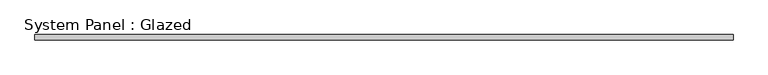
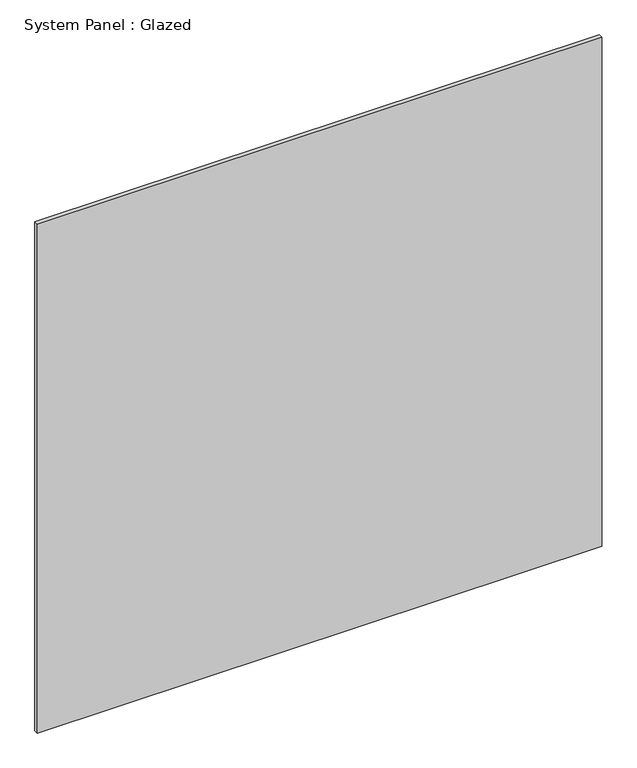
"""IFC4 building model written with IfcOpenShell, lengths in millimetres: plate geometry, System Panel : Glazed."""

from ifc_helpers import new_model, si_unit, origin, origin_with_axes, place, context, project, spatial, polyline, outline, extrude, source, transform, mapped, element, save


def system_panel_glazed_df7e0718(model_context):
    return source(origin(), model_context, "Body", "SweptSolid", [
        extrude(outline(polyline([(1573.2492557, 24.5), (-1573.2492557, 24.5), (-1573.2492557, 49.5), (1573.2492557, 49.5), (1573.2492557, 24.5)])), origin_with_axes(), (0.0, 0.0, 1.0), 3000.0),
    ])


if __name__ == "__main__":
    model = new_model("IFC4")
    model_context = context("Model", 3, world=origin())
    ifc_project = project(units=[si_unit("LENGTHUNIT", "METRE", prefix="MILLI")], contexts=[model_context])
    site = spatial("IfcSite", under=ifc_project)
    building = spatial("IfcBuilding", under=site)
    placement = place(None, origin())
    system_panel_glazed_shape = system_panel_glazed_df7e0718(model_context)
    element("IfcPlate", 1, ObjectType="System Panel : Glazed", at=placement, inside=building, context=model_context, shape_type="MappedRepresentation", body=[
        mapped(system_panel_glazed_shape, transform((0.0, 0.0, 0.0), x_axis=(1.0, 0.0, 0.0), y_axis=(0.0, 1.0, 0.0), z_axis=(0.0, 0.0, 1.0))),
    ])
    save(model, "model.ifc")

# Revit data of these elements
# Type "System Panel : Glazed"
#   Keynote = "H11"
#   Construction Type Id = "GSP4R"
#   Analytic Construction = "1/8 in Pilkington single glazing"
#   Visual Light Transmittance = 0.9
#   Solar Heat Gain Coefficient = 0.86
#   Heat Transfer Coefficient (U) = 6.7069 W/(m²·K)
#   Define Thermal Properties by = 1
# Element 1 (IfcPlate, "System Panel : Glazed")
#   Materials on its faces: "Glass"
# Materials
#   "Glass": class "Glass", colour RGB 0 128 192, transparency 0.9, Description = "Soda Lime Glass", Cost = 0
